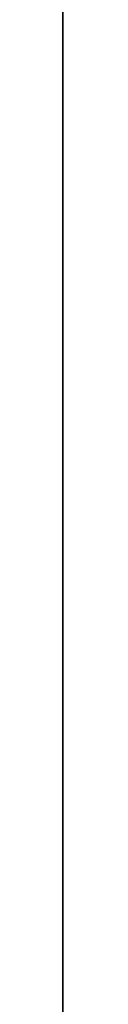
# Model space of a CAD drawing. Units: inches. Extents: x 2083 to 3317, y 1141 to 2115.
# Tile 34 of 256: x 2235.95977 to 2235.95984, y 1477.8005 to 1477.82142. Entities that reach past the tile are written whole.
import ezdxf

# ---------------------------------------------------------------- set-up
doc = ezdxf.new("R2010")
doc.units = ezdxf.units.IN
doc.layers.add('A-ANNO-DIMS', color=2, linetype='Continuous', lineweight=18)
doc.layers.add('A-WALL', color=7, linetype='Continuous', lineweight=35)
doc.layers.add('A-WALL-PATT', color=251, linetype='Continuous', lineweight=13, true_color=0x636466)
doc.styles.get("Standard").update_dxf_attribs({"font": 'arial.ttf'})
doc.dimstyles.new('ISO-25', dxfattribs={"dimtxt": 12, "dimasz": 12, "dimexe": 1.25, "dimexo": 0.625, "dimtad": 1, "dimlunit": 3, "dimtxsty": 'Standard', "dimcen": 2.5, "dimadec": 0, "dimazin": 0, "dimtfac": 1, "dimtmove": 0, "dimatfit": 3, "dimfxl": 1, "dimarcsym": 0})

# ---------------------------------------------------------------- blocks, each defined once
blk = doc.blocks.new('*D30')
at = {"layer": 'A-ANNO-DIMS', "color": 0, "lineweight": -2, "transparency": 16777216}
for p, q in [((2240.017856, 1445.273807), (2240.017856, 1448.045528)), ((2254.329327, 1445.273807), (2254.329327, 1448.045528)), ((2228.017856, 1446.795528), (2216.017856, 1446.795528)), ((2240.017856, 1446.795528), (2254.329327, 1446.795528)), ((2266.329327, 1446.795528), (2413.764866, 1446.795528))]:
    blk.add_line(p, q, dxfattribs=at)
at = {"layer": 'A-ANNO-DIMS', "color": 0, "transparency": 16777216}
for points in [[(2228.017856, 1448.795528), (2228.017856, 1444.795528), (2240.017856, 1446.795528)], [(2266.329327, 1448.795528), (2266.329327, 1444.795528), (2254.329327, 1446.795528)]]:
    blk.add_solid(points, dxfattribs=at)
at = {"layer": 'Defpoints', "color": 0, "transparency": 16777216}
for p in [(2254.329327, 1446.795528), (2240.017856, 1444.648807), (2254.329327, 1444.648807)]:
    blk.add_point(p, dxfattribs=at)
at = {"layer": 'A-ANNO-DIMS', "color": 0, "transparency": 16777216, "insert": (2346.047096, 1453.625167), "char_height": 12, "attachment_point": 5}
blk.add_mtext('WC 1\'-2 1/2" TYP.', dxfattribs=at)
blk = doc.blocks.new('*D31')
at = {"layer": 'A-ANNO-DIMS', "color": 0, "lineweight": -2, "transparency": 16777216}
for p, q in [((2237.871136, 1456.648807), (2237.871136, 1541.915179)), ((2239.392856, 1444.648807), (2236.621136, 1444.648807)), ((2237.871136, 1431.547542), (2237.871136, 1444.648807)), ((2239.392856, 1431.547542), (2236.621136, 1431.547542)), ((2237.871136, 1419.547542), (2237.871136, 1407.547542))]:
    blk.add_line(p, q, dxfattribs=at)
at = {"layer": 'A-ANNO-DIMS', "color": 0, "transparency": 16777216}
for points in [[(2235.871136, 1456.648807), (2239.871136, 1456.648807), (2237.871136, 1444.648807)], [(2235.871136, 1419.547542), (2239.871136, 1419.547542), (2237.871136, 1431.547542)]]:
    blk.add_solid(points, dxfattribs=at)
at = {"layer": 'Defpoints', "color": 0, "transparency": 16777216}
for p in [(2237.871136, 1444.648807), (2240.017856, 1444.648807), (2240.017856, 1431.547542)]:
    blk.add_point(p, dxfattribs=at)
at = {"layer": 'A-ANNO-DIMS', "color": 0, "transparency": 16777216, "insert": (2231.217486, 1505.281993), "char_height": 12, "attachment_point": 5, "rotation": 90}
blk.add_mtext('1\'-1" TYP.', dxfattribs=at)
blk = doc.blocks.new('*D45')
at = {"layer": 'A-ANNO-DIMS', "color": 0, "lineweight": -2, "transparency": 16777216}
for p, q in [((2235.959783, 1478.38636), (2235.959783, 1531.36136)), ((2418.959783, 1478.38636), (2418.959783, 1531.36136)), ((2247.959783, 1530.11136), (2406.959783, 1530.11136))]:
    blk.add_line(p, q, dxfattribs=at)
at = {"layer": 'A-ANNO-DIMS', "color": 0, "transparency": 16777216}
for points in [[(2247.959783, 1532.11136), (2247.959783, 1528.11136), (2235.959783, 1530.11136)], [(2406.959783, 1532.11136), (2406.959783, 1528.11136), (2418.959783, 1530.11136)]]:
    blk.add_solid(points, dxfattribs=at)
at = {"layer": 'Defpoints', "color": 0, "transparency": 16777216}
for p in [(2418.959783, 1530.11136), (2235.959783, 1477.76136), (2418.959783, 1477.76136)]:
    blk.add_point(p, dxfattribs=at)
at = {"layer": 'A-ANNO-DIMS', "color": 0, "transparency": 16777216, "insert": (2327.459783, 1536.867329), "char_height": 12, "attachment_point": 5}
blk.add_mtext('15\'-3"', dxfattribs=at)
blk = doc.blocks.new('*D62')
at = {"layer": 'A-ANNO-DIMS', "color": 0, "lineweight": -2, "transparency": 16777216}
for p, q in [((2235.959783, 1469.38636), (2235.959783, 1522.36136)), ((2379.959783, 1469.38636), (2379.959783, 1522.36136)), ((2247.959783, 1521.11136), (2367.959783, 1521.11136))]:
    blk.add_line(p, q, dxfattribs=at)
at = {"layer": 'A-ANNO-DIMS', "color": 0, "transparency": 16777216}
for points in [[(2247.959783, 1523.11136), (2247.959783, 1519.11136), (2235.959783, 1521.11136)], [(2367.959783, 1523.11136), (2367.959783, 1519.11136), (2379.959783, 1521.11136)]]:
    blk.add_solid(points, dxfattribs=at)
at = {"layer": 'Defpoints', "color": 0, "transparency": 16777216}
for p in [(2379.959783, 1521.11136), (2235.959783, 1468.76136), (2379.959783, 1468.76136)]:
    blk.add_point(p, dxfattribs=at)
at = {"layer": 'A-ANNO-DIMS', "color": 0, "transparency": 16777216, "insert": (2307.959783, 1527.863236), "char_height": 12, "attachment_point": 5}
blk.add_mtext('12\'-0"', dxfattribs=at)

msp = doc.modelspace()

# ---------------------------------------------------------------- hatches: boundary and pattern name
at = {"layer": 'A-WALL-PATT'}
h = msp.add_hatch(color=256, dxfattribs=at)
h.dxf.hatch_style = 1
h.paths.add_polyline_path([(3126.959783, 2020.76136), (2748.959783, 2020.76136), (2604.959783, 2020.76136), (2226.959783, 2020.76136), (2226.959783, 1702.76136), (2466.959783, 1702.76136), (2466.959783, 1582.76136), (2418.959783, 1582.76136), (2418.959783, 1477.76136), (2226.959783, 1477.76136), (2226.959783, 1263.26136), (2544.959783, 1263.26136), (2544.959783, 1411.76136), (2604.959783, 1411.76136), (2685.959783, 1411.76136), (2685.959783, 1420.76136), (2604.959783, 1420.76136), (2604.959783, 1573.76136), (2604.959783, 1702.76136), (2604.959783, 2011.76136), (2748.959783, 2011.76136), (2748.959783, 1702.76136), (2862.959783, 1702.76136), (2862.959783, 1621.76136), (2871.959783, 1621.76136), (2871.959783, 1702.76136), (2883.959783, 1702.76136), (2883.959783, 1706.939459, -0.026459), (2883.959783, 1711.76136), (2757.959783, 1711.76136), (2757.959783, 1807.76136), (2787.959783, 1807.76136), (2787.959783, 1812.26136), (2757.959783, 1812.26136), (2757.959783, 2011.76136), (2877.959783, 2011.76136), (2877.959783, 1812.26136), (2847.959783, 1812.26136), (2847.959783, 1807.76136), (2889.835742, 1807.76136), (2889.835742, 1812.26136), (2882.459783, 1812.26136), (2882.459783, 2011.76136), (3117.959783, 2011.76136), (3117.959783, 1812.26136), (2937.835742, 1812.26136), (2937.835742, 1807.76136), (2995.709783, 1807.76136), (2995.709783, 1796.117666), (3000.209783, 1796.117666), (3000.209783, 1807.76136), (3117.959783, 1807.76136), (3117.959783, 1711.76136), (3000.209783, 1711.76136), (3000.209783, 1760.117666), (2998.572705, 1760.117666, -0.020711), (2995.709783, 1760.117666), (2995.709783, 1711.76136), (2931.959783, 1711.76136), (2931.959783, 1702.76136), (3126.959783, 1702.76136)])
h.paths.add_polyline_path([(2471.459783, 2011.76136), (2471.459783, 1810.01136), (2462.716936, 1810.01136), (2462.716936, 1805.51136), (2505.959783, 1805.51136), (2505.959783, 1810.01136), (2475.959783, 1810.01136), (2475.959783, 2011.76136), (2595.959783, 2011.76136), (2595.959783, 1810.01136), (2565.959783, 1810.01136), (2565.959783, 1805.51136), (2595.959783, 1805.51136), (2595.959783, 1711.76136), (2235.959783, 1711.76136), (2235.959783, 1805.51136), (2353.709783, 1805.51136), (2353.709783, 1796.054162), (2358.209783, 1796.054162), (2358.209783, 1805.51136), (2414.716936, 1805.51136), (2414.716936, 1810.01136), (2235.959783, 1810.01136), (2235.959783, 2011.76136)], flags=16)
h.paths.add_polyline_path([(2270.204734, 1994.610008), (2270.204734, 1970.610008), (2246.204734, 1970.610008), (2246.204734, 1994.610008)], flags=0)
edge = h.paths.add_edge_path(flags=0)
edge.add_ellipse((2332.027391, 1899.798176), major_axis=(-3.042994, 3.042994), ratio=0.16825245, start_angle=-161.332166, end_angle=-156.307114, ccw=False)
edge.add_ellipse((2333.082037, 1898.74353), major_axis=(-1.054646, 1.054646), ratio=0.4535321, start_angle=-123.371019, end_angle=-94.159107)
edge = h.paths.add_edge_path(flags=0)
edge.add_ellipse((2332.027391, 1968.87629), major_axis=(3.042994, 3.042994), ratio=0.16825245, start_angle=18.667834, end_angle=23.692886)
edge.add_spline(control_points=[(2332.925596, 1970.691105), (2332.226768, 1970.3361), (2330.893709, 1969.658905), (2328.41308, 1970.932138), (2327.203934, 1967.748712), (2324.709596, 1969.955589), (2322.532822, 1967.012354), (2320.012846, 1971.295812), (2317.680308, 1968.157845), (2316.040526, 1967.102047), (2315.426904, 1966.809602)], knot_values=[0, 0, 0, 0, 2.267059, 4.324559, 6.685584, 8.878641, 11.121502, 14.300359, 17.755284, 19.732645, 19.732645, 19.732645, 19.732645], degree=3, periodic=0)
edge.add_ellipse((2332.027391, 1968.87629), major_axis=(3.042994, 3.042994), ratio=0.16825245, start_angle=18.667834, end_angle=23.692886, ccw=False)
edge.add_ellipse((2333.082037, 1969.930936), major_axis=(1.054646, 1.054646), ratio=0.4535321, start_angle=56.628981, end_angle=85.840893, ccw=False)
edge = h.paths.add_edge_path(flags=0)
edge.add_spline(control_points=[(2296.428287, 1967.987908), (2293.627804, 1965.336314), (2287.703624, 1959.727094), (2299.74386, 1949.995699), (2294.532591, 1935.668528), (2290.573228, 1920.603512), (2293.394124, 1909.973691), (2296.185407, 1904.966543)], knot_values=[0.099185, 0.099185, 0.099185, 0.099185, 0.345301, 0.619822, 0.982653, 1.386093, 1.810555, 1.810555, 1.810555, 1.810555], degree=3, periodic=0)
edge.add_spline(control_points=[(2296.185407, 1904.966543), (2297.383582, 1902.6193), (2298.000969, 1901.949312), (2298.55297, 1901.468155)], knot_values=[0.006246, 0.006246, 0.006246, 0.006246, 0.055476, 0.055476, 0.055476, 0.055476], degree=3, periodic=0)
edge.add_spline(control_points=[(2298.55297, 1901.468155), (2297.258612, 1900.923224), (2295.225294, 1900.232126), (2293.060229, 1900.614205), (2292.101423, 1900.788415), (2292.089578, 1900.790568)], knot_values=[0.312835, 0.312835, 0.312835, 0.312835, 0.40178, 0.474987, 0.475903, 0.475903, 0.475903, 0.475903], degree=3, periodic=0)
edge.add_arc((2292.793646, 1904.664109), 3.937008, 215.420897, 259.698179, ccw=False)
edge.add_spline(control_points=[(2289.585314, 1902.382304), (2289.476652, 1902.535087), (2289.36848, 1902.688035), (2289.260865, 1902.84117)], knot_values=[0.102872, 0.102872, 0.102872, 0.102872, 0.116896, 0.116896, 0.116896, 0.116896], degree=3, periodic=0)
edge.add_spline(control_points=[(2289.260865, 1902.84117), (2288.686604, 1902.550192), (2287.640048, 1902.019902), (2285.881337, 1901.873954), (2283.852972, 1901.504352), (2281.719987, 1899.710538), (2278.466991, 1899.492942), (2276.157136, 1901.883202), (2272.258953, 1899.804071), (2267.777605, 1901.843183), (2262.243882, 1900.184033), (2257.414927, 1901.782061), (2254.318374, 1900.72612), (2253.178285, 1900.337343)], knot_values=[0, 0, 0, 0, 1.907977, 3.477176, 5.261074, 7.972851, 11.680248, 13.717921, 16.939592, 22.789562, 27.502503, 33.595215, 37.145618, 37.145618, 37.145618, 37.145618], degree=3, periodic=0)
edge.add_line((2253.178285, 1900.337343), (2250.24424, 1902.84117))
edge.add_line((2250.24424, 1902.84117), (2250.24424, 1965.833296))
edge.add_line((2250.24424, 1965.833296), (2253.178285, 1968.337123))
edge.add_spline(control_points=[(2253.178285, 1968.337123), (2254.318374, 1967.948346), (2257.414927, 1966.892405), (2262.243882, 1968.490433), (2267.777605, 1966.831283), (2271.52673, 1968.537217), (2273.875914, 1967.828289), (2274.206701, 1967.727642)], knot_values=[0, 0, 0, 0, 0.09018, 0.244935, 0.364644, 0.513233, 0.537855, 0.537855, 0.537855, 0.537855], degree=3, periodic=0)
edge.add_arc((2274.352887, 1963.793349), 3.937008, 72.051134, 92.127949, ccw=False)
edge.add_arc((2281.296933, 1985.230003), 18.596298, 252.0511336, 288.5657217)
edge.add_arc((2292.316717, 1956.02888), 12.646081, 71.0267879, 113.7782184, ccw=False)
edge = h.paths.add_edge_path(flags=0)
edge.add_spline(control_points=[(2274.899415, 1951.856195), (2275.066156, 1951.616592), (2275.232687, 1951.376588), (2275.397987, 1951.135855)], knot_values=[1.409916, 1.409916, 1.409916, 1.409916, 1.43159, 1.43159, 1.43159, 1.43159], degree=3, periodic=0)
edge.add_spline(control_points=[(2275.397987, 1951.135855), (2275.792106, 1950.561885), (2276.179231, 1949.983774), (2276.545546, 1949.397103)], knot_values=[1.358238, 1.358238, 1.358238, 1.358238, 1.409916, 1.409916, 1.409916, 1.409916], degree=3, periodic=0)
edge.add_line((2276.545546, 1949.397103), (2277.437289, 1947.862185))
edge.add_spline(control_points=[(2277.437289, 1947.862185), (2276.303834, 1945.673115), (2274.639698, 1942.426882), (2274.631615, 1938.0939), (2272.799124, 1930.85155), (2274.356426, 1943.897046), (2275.947681, 1947.923356), (2276.545546, 1949.397103)], knot_values=[0.005632, 0.005632, 0.005632, 0.005632, 0.186014, 0.266002, 0.357087, 0.59639, 0.739732, 0.739732, 0.739732, 0.739732], degree=3, periodic=0)
edge.add_spline(control_points=[(2276.545546, 1949.397103), (2276.179231, 1949.983774), (2275.792106, 1950.561885), (2275.397987, 1951.135855)], knot_values=[1.358238, 1.358238, 1.358238, 1.358238, 1.409916, 1.409916, 1.409916, 1.409916], degree=3, periodic=0)
edge.add_spline(control_points=[(2275.397987, 1951.135855), (2274.9425, 1950.080452), (2274.20776, 1948.025272), (2273.934602, 1944.851477), (2272.468534, 1937.627489), (2273.466216, 1945.696466), (2274.700615, 1951.059472), (2274.899415, 1951.856195)], knot_values=[0.104364, 0.104364, 0.104364, 0.104364, 0.189636, 0.269624, 0.36071, 0.600013, 0.644622, 0.644622, 0.644622, 0.644622], degree=3, periodic=0)
h.paths.add_polyline_path([(2269.167514, 1963.127573, -0.357527), (2268.170633, 1960.97637, -0.092561), (2268.170633, 1939.436325, -0.357527), (2269.167514, 1937.285122, -0.357527), (2267.01631, 1938.282002, -0.164785), (2254.685581, 1938.282002, -0.357527), (2252.534378, 1937.285122, -0.357527), (2253.531259, 1939.436325, -0.092561), (2253.531259, 1960.97637, -0.357527), (2252.534378, 1963.127573, -0.357527), (2254.685581, 1962.130692, -0.164785), (2267.01631, 1962.130692, -0.357527)], flags=0)
h.paths.add_polyline_path([(2248.874068, 1967.8018), (2248.874068, 1957.02771), (2249.457783, 1957.02771), (2249.457783, 1911.646756), (2248.874068, 1911.646756), (2248.874068, 1900.872666), (2246.511863, 1900.872666, 0.197327), (2244.149658, 1902.456873), (2244.149658, 1966.217592, 0.197327), (2246.511863, 1967.8018)], flags=0)
h.paths.add_polyline_path([(2269.167514, 1931.389344, -0.357527), (2268.170633, 1929.238141, -0.092561), (2268.170633, 1907.698096, -0.357527), (2269.167514, 1905.546893, -0.357527), (2267.01631, 1906.543774, -0.164785), (2254.685581, 1906.543774, -0.357527), (2252.534378, 1905.546893, -0.357527), (2253.531259, 1907.698096, -0.092561), (2253.531259, 1929.238141, -0.357527), (2252.534378, 1931.389344, -0.357527), (2254.685581, 1930.392463, -0.164785), (2267.01631, 1930.392463, -0.357527)], flags=0)
edge = h.paths.add_edge_path(flags=0)
edge.add_spline(control_points=[(2276.196858, 1906.723702), (2276.168144, 1909.028928), (2276.114049, 1913.371852), (2270.598417, 1924.924978), (2273.905175, 1919.012779), (2275.921711, 1916.262063), (2275.47457, 1912.402149), (2277.257874, 1910.380621), (2276.696044, 1908.225036), (2276.646218, 1906.813023), (2276.617825, 1906.008407)], knot_values=[0, 0, 0, 0, 8.61026, 16.221274, 18.843057, 23.804898, 27.440828, 29.356102, 31.203478, 33.650687, 33.650687, 33.650687, 33.650687], degree=3, periodic=0)
edge.add_spline(control_points=[(2276.617825, 1906.008407), (2276.623313, 1905.624144), (2276.497738, 1904.628661), (2275.441779, 1903.854725), (2274.937314, 1903.08045), (2274.85908, 1902.84117)], knot_values=[0.156488, 0.156488, 0.156488, 0.156488, 0.184398, 0.231376, 0.250598, 0.250598, 0.250598, 0.250598], degree=3, periodic=0)
edge.add_line((2274.85908, 1902.84117), (2276.50598, 1902.84117))
edge.add_spline(control_points=[(2276.50598, 1902.84117), (2276.788308, 1903.08494), (2277.665071, 1904.125196), (2278.249538, 1904.340738), (2277.653872, 1908.527387), (2278.15567, 1906.227808), (2278.100464, 1905.285948), (2278.846675, 1904.069005), (2277.856785, 1903.414948), (2277.874191, 1902.99105), (2277.903562, 1902.84117)], knot_values=[0.059574, 0.059574, 0.059574, 0.059574, 0.080753, 0.103741, 0.16972, 0.176036, 0.207137, 0.240474, 0.262341, 0.27366, 0.27366, 0.27366, 0.27366], degree=3, periodic=0)
edge.add_line((2277.903562, 1902.84117), (2280.029825, 1902.84117))
edge.add_spline(control_points=[(2280.029825, 1902.84117), (2279.888221, 1903.088398), (2279.499257, 1903.981551), (2280.152284, 1905.939349), (2278.103615, 1909.657757), (2279.762395, 1907.185285), (2280.3279, 1904.874861), (2280.485109, 1903.48959), (2281.463269, 1903.249432), (2281.758343, 1902.936497), (2281.834036, 1902.84117)], knot_values=[0.013856, 0.013856, 0.013856, 0.013856, 0.034874, 0.088867, 0.107879, 0.126738, 0.158714, 0.193757, 0.217487, 0.226722, 0.226722, 0.226722, 0.226722], degree=3, periodic=0)
edge.add_spline(control_points=[(2281.834036, 1902.84117), (2281.787535, 1902.826703), (2281.647022, 1902.782988), (2281.395527, 1902.85949), (2281.088077, 1902.985242), (2280.720683, 1903.060902), (2280.333451, 1903.025726), (2280.124767, 1902.898879), (2280.029825, 1902.84117)], knot_values=[0, 0, 0, 0, 0.14413, 0.435517, 0.749276, 1.153046, 1.548371, 1.878348, 1.878348, 1.878348, 1.878348], degree=3, periodic=0)
edge.add_line((2280.029825, 1902.84117), (2277.903562, 1902.84117))
edge.add_spline(control_points=[(2277.903562, 1902.84117), (2277.892855, 1902.795855), (2277.865396, 1902.679637), (2277.607479, 1902.687483), (2277.27405, 1902.8007), (2276.837921, 1902.619775), (2276.583807, 1902.789261), (2276.50598, 1902.84117)], knot_values=[0, 0, 0, 0, 0.127189, 0.326199, 0.628009, 1.24357, 1.515331, 1.515331, 1.515331, 1.515331], degree=3, periodic=0)
edge.add_line((2276.50598, 1902.84117), (2274.85908, 1902.84117))
edge.add_spline(control_points=[(2274.85908, 1902.84117), (2274.814437, 1902.898587), (2274.72513, 1903.013446), (2274.493477, 1903.118968), (2274.244285, 1902.960539), (2273.937121, 1903.184942), (2273.614039, 1902.983143), (2273.408316, 1902.883045), (2273.322254, 1902.84117)], knot_values=[0, 0, 0, 0, 0.21843, 0.436957, 0.687977, 0.990379, 1.398396, 1.69185, 1.69185, 1.69185, 1.69185], degree=3, periodic=0)
edge.add_spline(control_points=[(2273.322254, 1902.84117), (2273.61674, 1903.445692), (2274.273998, 1904.538253), (2276.027239, 1904.573702), (2276.206963, 1906.583637), (2276.196858, 1906.723702)], knot_values=[0.012227, 0.012227, 0.012227, 0.012227, 0.059472, 0.106218, 0.134458, 0.134458, 0.134458, 0.134458], degree=3, periodic=0)
h.paths.add_polyline_path([(2270.776054, 1897.789828), (2270.776054, 1873.789828), (2246.776054, 1873.789828), (2246.776054, 1897.789828)], flags=0)
h.paths.add_polyline_path([(2353.709783, 1760.005059), (2353.709783, 1760.054162), (2358.209783, 1760.054162, -0.033729)], flags=0)
h.paths.add_polyline_path([(2321.819119, 1737.529186), (2341.995327, 1737.529186, -0.414214), (2343.203273, 1736.321241), (2343.203273, 1721.020596, -0.414214), (2341.995327, 1719.812651), (2321.819119, 1719.812651, -0.414214), (2320.611173, 1721.020596), (2320.611173, 1736.321241, -0.414214)], flags=0)
h.paths.add_polyline_path([(2324.23501, 1736.321241), (2339.579436, 1736.321241, -0.414214), (2341.995327, 1733.905349), (2341.995327, 1725.44973, -0.414214), (2339.579436, 1723.033839), (2333.680588, 1723.033839), (2333.845317, 1722.045467, -0.870646), (2335.425399, 1721.825893, -0.767327), (2333.922694, 1721.423245), (2331.291024, 1721.423245, -0.767327), (2329.788319, 1721.825893, -0.870646), (2331.368401, 1722.045467), (2331.53313, 1723.033839), (2324.23501, 1723.033839, -0.414214), (2321.819119, 1725.44973), (2321.819119, 1733.905349, -0.414214)], flags=0)
h.paths.add_polyline_path([(2570.483789, 1928.615444), (2589.683789, 1928.615444), (2590.168829, 1928.615444), (2590.168829, 1904.993397), (2570.483789, 1904.993397)], flags=0)
h.paths.add_polyline_path([(2574.447324, 1927.263822, -1), (2572.828836, 1927.263822, -1)], flags=0)
h.paths.add_polyline_path([(2573.089867, 1926.940877), (2573.925032, 1927.776042), (2574.147743, 1927.553332), (2573.312577, 1926.718166)], flags=0)
h.paths.add_polyline_path([(2578.779065, 1919.729618, -1), (2571.591663, 1919.729618, -1)], flags=0)
h.paths.add_polyline_path([(2578.385364, 1919.729618, -1), (2571.985364, 1919.729618, -1)], flags=0)
h.paths.add_polyline_path([(2331.595764, 1729.476216, -1), (2333.617954, 1729.476216, -1)], flags=0)
h.paths.add_polyline_path([(2578.034228, 1927.263822, -1), (2576.41574, 1927.263822, -1)], flags=0)
h.paths.add_polyline_path([(2576.688851, 1927.531089), (2576.911562, 1927.753799), (2577.746728, 1926.918634), (2577.524017, 1926.695923)], flags=0)
h.paths.add_polyline_path([(2578.139065, 1909.859539, -1), (2572.231663, 1909.859539, -1)], flags=0)
h.paths.add_polyline_path([(2577.745364, 1909.859539, -1), (2572.625364, 1909.859539, -1)], flags=0)
h.paths.add_polyline_path([(2583.797718, 1927.263822, -1), (2582.179229, 1927.263822, -1)], flags=0)
h.paths.add_polyline_path([(2582.718649, 1927.753799), (2583.553814, 1926.918634), (2583.331103, 1926.695923), (2582.495938, 1927.531089)], flags=0)
h.paths.add_polyline_path([(2582.495938, 1927.531089), (2582.718649, 1927.753799), (2583.553814, 1926.918634), (2583.331103, 1926.695923)], flags=0)
h.paths.add_polyline_path([(2587.739065, 1920.529618, -1), (2581.831663, 1920.529618, -1)], flags=0)
h.paths.add_polyline_path([(2587.345364, 1920.529618, -1), (2582.225364, 1920.529618, -1)], flags=0)
h.paths.add_polyline_path([(2587.384622, 1927.263822, -1), (2585.766133, 1927.263822, -1)], flags=0)
h.paths.add_polyline_path([(2586.081993, 1926.980247), (2586.917158, 1927.815412), (2587.139869, 1927.592702), (2586.304703, 1926.757536)], flags=0)
h.paths.add_polyline_path([(2588.379065, 1910.659539, -1), (2581.191663, 1910.659539, -1)], flags=0)
h.paths.add_polyline_path([(2587.985364, 1910.659539, -1), (2581.585364, 1910.659539, -1)], flags=0)
h.paths.add_polyline_path([(2417.167729, 1729.477895), (2437.343937, 1729.477895, -0.414214), (2438.551883, 1728.26995), (2438.551883, 1712.969306, -0.414214), (2437.343937, 1711.76136), (2417.167729, 1711.76136, -0.414214), (2415.959783, 1712.969306), (2415.959783, 1728.26995, -0.414214)], flags=0)
h.paths.add_polyline_path([(2419.58362, 1728.26995), (2434.928046, 1728.26995, -0.414214), (2437.343937, 1725.854059), (2437.343937, 1717.39844, -0.414214), (2434.928046, 1714.982548), (2429.029199, 1714.982548), (2429.193927, 1713.994176, -0.870646), (2430.774009, 1713.774603, -0.767327), (2429.271304, 1713.371954), (2426.639634, 1713.371954, -0.767327), (2425.136929, 1713.774603, -0.870646), (2426.717011, 1713.994176), (2426.88174, 1714.982548), (2419.58362, 1714.982548, -0.414214), (2417.167729, 1717.39844), (2417.167729, 1725.854059, -0.414214)], flags=0)
h.paths.add_polyline_path([(2419.58362, 1728.26995), (2434.928046, 1728.26995, -0.414214), (2437.343937, 1725.854059), (2437.343937, 1717.39844, -0.414214), (2434.928046, 1714.982548), (2429.029199, 1714.982548), (2428.358118, 1719.009034), (2427.552821, 1719.009034), (2426.88174, 1714.982548), (2419.58362, 1714.982548, -0.414214), (2417.167729, 1717.39844), (2417.167729, 1725.854059, -0.414214)], flags=0)
h.paths.add_polyline_path([(2426.944374, 1721.424925, -1), (2428.966564, 1721.424925, -1)], flags=0)
h.paths.add_polyline_path([(2475.959783, 1702.76136), (2595.959783, 1702.76136), (2595.959783, 1582.76136), (2475.959783, 1582.76136)], flags=16)
h.paths.add_polyline_path([(2427.959783, 1573.76136), (2595.959783, 1573.76136), (2595.959783, 1468.76136), (2595.959783, 1420.76136), (2384.459783, 1420.76136), (2384.459783, 1468.76136), (2427.959783, 1468.76136)], flags=16)
h.paths.add_polyline_path([(2379.959783, 1468.76136), (2379.959783, 1420.76136), (2235.959783, 1420.76136), (2235.959783, 1468.76136)], flags=16)
h.paths.add_polyline_path([(2317.815996, 1466.695767), (2337.992205, 1466.695767, -0.414214), (2339.20015, 1465.487821), (2339.20015, 1450.187177, -0.414214), (2337.992205, 1448.979232), (2317.815996, 1448.979232, -0.414214), (2316.608051, 1450.187177), (2316.608051, 1465.487821, -0.414214)], flags=0)
h.paths.add_polyline_path([(2320.231887, 1465.487821), (2335.576313, 1465.487821, -0.414214), (2337.992205, 1463.07193), (2337.992205, 1454.616311, -0.414214), (2335.576313, 1452.20042), (2329.677466, 1452.20042), (2329.842195, 1451.212047, -0.870646), (2331.422276, 1450.992474, -0.767327), (2329.919571, 1450.589826), (2327.287902, 1450.589826, -0.767327), (2325.785197, 1450.992474, -0.870646), (2327.365278, 1451.212047), (2327.530007, 1452.20042), (2320.231887, 1452.20042, -0.414214), (2317.815996, 1454.616311), (2317.815996, 1463.07193, -0.414214)], flags=0)
h.paths.add_polyline_path([(2320.231887, 1465.487821), (2335.576313, 1465.487821, -0.414214), (2337.992205, 1463.07193), (2337.992205, 1454.616311, -0.414214), (2335.576313, 1452.20042), (2329.677466, 1452.20042), (2329.006385, 1456.226905), (2328.201088, 1456.226905), (2327.530007, 1452.20042), (2320.231887, 1452.20042, -0.414214), (2317.815996, 1454.616311), (2317.815996, 1463.07193, -0.414214)], flags=0)
h.paths.add_polyline_path([(2327.592641, 1458.642796, -1), (2329.614832, 1458.642796, -1)], flags=0)
h.paths.add_polyline_path([(2244.411744, 1433.340453), (2241.920945, 1433.340453, -0.414214), (2240.017856, 1435.243542), (2240.017856, 1440.952808, -0.414211), (2241.920925, 1442.855897), (2244.411744, 1442.855897, -1.976472)], flags=0)
h.paths.add_polyline_path([(2245.356888, 1434.397536, -0.414214), (2245.356888, 1441.798814, -2.144098)], flags=0)
h.paths.add_polyline_path([(2535.959783, 1416.26136), (2535.959783, 1272.26136), (2235.959783, 1272.26136), (2235.959783, 1416.26136)], flags=16)
h.paths.add_polyline_path([(2260.119561, 1384.292841), (2260.119561, 1362.038649), (2237.865369, 1362.038649), (2237.865369, 1384.292841)], flags=0)
edge = h.paths.add_edge_path(flags=0)
edge.add_line((2318.251847, 1362.093298), (2318.145797, 1362.000973))
edge.add_ellipse((2317.445116, 1360.431044), major_axis=(2.82164, 2.82164), ratio=0.16825245, start_angle=18.667834, end_angle=20.948127, ccw=False)
edge.add_ellipse((2318.423045, 1361.408974), major_axis=(0.977929, 0.977929), ratio=0.4535321, start_angle=56.628981, end_angle=70.226201, ccw=False)
edge = h.paths.add_edge_path(flags=0)
edge.add_line((2319.10737, 1295.571078), (2319.015044, 1295.677128))
edge.add_ellipse((2317.445116, 1296.377809), major_axis=(-2.82164, 2.82164), ratio=0.16825245, start_angle=-161.332166, end_angle=-159.051873, ccw=False)
edge.add_ellipse((2318.423045, 1295.39988), major_axis=(-0.977929, 0.977929), ratio=0.4535321, start_angle=-123.371019, end_angle=-109.773799)
edge = h.paths.add_edge_path(flags=0)
edge.add_spline(control_points=[(2284.210349, 1301.170219), (2284.580688, 1300.444719), (2284.891189, 1299.892024), (2285.159553, 1299.461018)], knot_values=[0.039066, 0.039066, 0.039066, 0.039066, 0.055476, 0.055476, 0.055476, 0.055476], degree=3, periodic=0)
edge.add_line((2285.159553, 1299.461018), (2284.210349, 1301.170219))
edge = h.paths.add_edge_path(flags=0)
edge.add_line((2280.412458, 1297.298013), (2283.369991, 1297.036122))
edge.add_line((2283.369991, 1297.036122), (2286.40569, 1297.92631))
edge.add_spline(control_points=[(2286.40569, 1297.92631), (2285.305487, 1297.463119), (2284.344777, 1297.129151), (2283.369991, 1297.036122)], knot_values=[0.394369, 0.394369, 0.394369, 0.394369, 0.475903, 0.475903, 0.475903, 0.475903], degree=3, periodic=0)
edge.add_spline(control_points=[(2283.369991, 1297.036122), (2283.28139, 1297.027666), (2282.316289, 1296.957336), (2281.312502, 1297.134479), (2280.423441, 1297.296016), (2280.412458, 1297.298013)], knot_values=[0.312835, 0.312835, 0.312835, 0.312835, 0.320246, 0.393453, 0.394369, 0.394369, 0.394369, 0.394369], degree=3, periodic=0)
edge = h.paths.add_edge_path(flags=0)
edge.add_line((2284.435561, 1359.607285), (2280.446291, 1355.328047))
edge.add_line((2280.446291, 1355.328047), (2279.579987, 1351.017754))
edge.add_line((2279.579987, 1351.017754), (2282.412974, 1346.580433))
edge.add_spline(control_points=[(2282.412974, 1346.580433), (2283.153331, 1345.589236), (2284.252896, 1344.028897), (2284.801037, 1342.387167), (2284.935162, 1341.805544)], knot_values=[1.240098, 1.240098, 1.240098, 1.240098, 1.332892, 1.382712, 1.382712, 1.382712, 1.382712], degree=3, periodic=0)
edge.add_spline(control_points=[(2284.935162, 1341.805544), (2285.319108, 1340.1406), (2285.233029, 1338.409204), (2284.909938, 1336.654122)], knot_values=[1.097484, 1.097484, 1.097484, 1.097484, 1.240098, 1.240098, 1.240098, 1.240098], degree=3, periodic=0)
edge.add_spline(control_points=[(2284.909938, 1336.654122), (2284.586848, 1334.89904), (2284.026745, 1333.120272), (2283.462644, 1331.360585)], knot_values=[0.95487, 0.95487, 0.95487, 0.95487, 1.097484, 1.097484, 1.097484, 1.097484], degree=3, periodic=0)
edge.add_line((2283.462644, 1331.360585), (2281.890376, 1326.153357))
edge.add_line((2281.890376, 1326.153357), (2280.756259, 1321.056089))
edge.add_line((2280.756259, 1321.056089), (2280.299205, 1316.001977))
edge.add_line((2280.299205, 1316.001977), (2280.715933, 1310.950068))
edge.add_line((2280.715933, 1310.950068), (2282.028094, 1305.972137))
edge.add_line((2282.028094, 1305.972137), (2284.210349, 1301.170219))
edge.add_spline(control_points=[(2284.210349, 1301.170219), (2283.340731, 1302.730185), (2282.611904, 1304.336493), (2282.028094, 1305.972137)], knot_values=[0.099185, 0.099185, 0.099185, 0.099185, 0.241799, 0.241799, 0.241799, 0.241799], degree=3, periodic=0)
edge.add_spline(control_points=[(2282.028094, 1305.972137), (2281.444283, 1307.60778), (2281.005489, 1309.272759), (2280.715933, 1310.950068)], knot_values=[0.241799, 0.241799, 0.241799, 0.241799, 0.384413, 0.384413, 0.384413, 0.384413], degree=3, periodic=0)
edge.add_spline(control_points=[(2280.715933, 1310.950068), (2280.433241, 1312.587613), (2280.289386, 1314.276959), (2280.298894, 1315.962032), (2280.299205, 1316.001977)], knot_values=[0.384413, 0.384413, 0.384413, 0.384413, 0.523647, 0.527028, 0.527028, 0.527028, 0.527028], degree=3, periodic=0)
edge.add_spline(control_points=[(2280.299205, 1316.001977), (2280.312326, 1317.686955), (2280.477871, 1319.367926), (2280.756259, 1321.056089)], knot_values=[0.527028, 0.527028, 0.527028, 0.527028, 0.669642, 0.669642, 0.669642, 0.669642], degree=3, periodic=0)
edge.add_spline(control_points=[(2280.756259, 1321.056089), (2281.034648, 1322.744252), (2281.42588, 1324.439608), (2281.890376, 1326.153357)], knot_values=[0.669642, 0.669642, 0.669642, 0.669642, 0.812256, 0.812256, 0.812256, 0.812256], degree=3, periodic=0)
edge.add_spline(control_points=[(2281.890376, 1326.153357), (2282.264383, 1327.533251), (2282.78787, 1329.26181), (2283.352751, 1331.01778), (2283.462644, 1331.360585)], knot_values=[0.812256, 0.812256, 0.812256, 0.812256, 0.927087, 0.95487, 0.95487, 0.95487, 0.95487], degree=3, periodic=0)
edge.add_line((2283.462644, 1331.360585), (2284.909938, 1336.654122))
edge.add_line((2284.909938, 1336.654122), (2284.935162, 1341.805544))
edge.add_line((2284.935162, 1341.805544), (2282.412974, 1346.580433))
edge.add_spline(control_points=[(2282.412974, 1346.580433), (2281.275127, 1348.103792), (2280.078447, 1349.570318), (2279.579987, 1351.017754)], knot_values=[1.382712, 1.382712, 1.382712, 1.382712, 1.525326, 1.525326, 1.525326, 1.525326], degree=3, periodic=0)
edge.add_spline(control_points=[(2279.579987, 1351.017754), (2279.443282, 1351.414721), (2279.136312, 1352.856922), (2279.73519, 1354.290385), (2280.446291, 1355.328047)], knot_values=[1.525326, 1.525326, 1.525326, 1.525326, 1.564439, 1.667941, 1.667941, 1.667941, 1.667941], degree=3, periodic=0)
edge.add_spline(control_points=[(2280.446291, 1355.328047), (2281.426113, 1356.757835), (2282.930837, 1358.18256), (2284.435561, 1359.607285)], knot_values=[1.667941, 1.667941, 1.667941, 1.667941, 1.810555, 1.810555, 1.810555, 1.810555], degree=3, periodic=0)
edge.add_arc((2280.623075, 1348.518181), 11.72618, 71.0267879, 113.7782184)
edge.add_arc((2270.404892, 1375.595156), 17.243567, 252.0511336, 288.5657217, ccw=False)
edge.add_arc((2263.965969, 1355.717847), 3.650622, 72.051134, 92.127949)
edge.add_arc((2263.965969, 1355.717847), 3.650622, 92.127949, 177.98513)
edge.add_spline(control_points=[(2260.317604, 1355.846199), (2260.260417, 1354.220668), (2260.551278, 1350.186547), (2262.999344, 1346.766251), (2264.472741, 1344.649024)], knot_values=[1.43159, 1.43159, 1.43159, 1.43159, 1.564144, 1.770695, 1.770695, 1.770695, 1.770695], degree=3, periodic=0)
edge.add_line((2264.472741, 1344.649024), (2264.93559, 1343.98253))
edge.add_spline(control_points=[(2263.801044, 1340.248105), (2263.843238, 1340.514088), (2264.067244, 1341.756465), (2264.512693, 1343.002453), (2264.935047, 1343.981083)], knot_values=[0.53657, 0.53657, 0.53657, 0.53657, 0.559349, 0.644622, 0.644622, 0.644622, 0.644622], degree=3, periodic=0)
edge.add_spline(control_points=[(2264.935047, 1343.981083), (2265.117771, 1343.714975), (2265.298875, 1343.447906), (2265.476756, 1343.179365)], knot_values=[1.384077, 1.384077, 1.384077, 1.384077, 1.409916, 1.409916, 1.409916, 1.409916], degree=3, periodic=0)
edge.add_spline(control_points=[(2265.476756, 1343.179365), (2265.654637, 1342.910823), (2265.829296, 1342.64081), (2265.99913, 1342.368812)], knot_values=[1.358238, 1.358238, 1.358238, 1.358238, 1.384077, 1.384077, 1.384077, 1.384077], degree=3, periodic=0)
edge.add_line((2265.99913, 1342.368812), (2266.826006, 1340.945547))
edge.add_spline(control_points=[(2266.826006, 1340.945547), (2268.894401, 1337.089691), (2271.398173, 1325.843001), (2270.516164, 1310.568557), (2275.919376, 1301.860609), (2277.789511, 1299.19945)], knot_values=[0.116896, 0.116896, 0.116896, 0.116896, 0.472987, 1.050969, 1.313793, 1.313793, 1.313793, 1.313793], degree=3, periodic=0)
edge.add_spline(control_points=[(2277.789511, 1299.19945), (2277.839405, 1299.128452), (2277.889428, 1299.057498), (2277.939572, 1298.986584)], knot_values=[0.109884, 0.109884, 0.109884, 0.109884, 0.116896, 0.116896, 0.116896, 0.116896], degree=3, periodic=0)
edge.add_line((2277.939572, 1298.986584), (2277.788849, 1299.199114))
edge.add_spline(control_points=[(2277.788849, 1299.199114), (2277.256582, 1298.929414), (2276.28635, 1298.437902), (2275.039352, 1298.334419), (2274.38333, 1298.238895), (2274.215254, 1298.209338)], knot_values=[33.12187, 33.12187, 33.12187, 33.12187, 35.029056, 36.598255, 37.144827, 37.144827, 37.144827, 37.144827], degree=3, periodic=0)
edge.add_line((2274.215254, 1298.209338), (2273.073147, 1297.892961))
edge.add_spline(control_points=[(2273.073147, 1297.892961), (2272.322936, 1297.579784), (2271.039151, 1296.510508), (2269.248395, 1296.226062), (2268.4231, 1296.374654)], knot_values=[26.532584, 26.532584, 26.532584, 26.532584, 29.198919, 31.839101, 31.839101, 31.839101, 31.839101], degree=3, periodic=0)
edge.add_line((2268.4231, 1296.374654), (2263.878501, 1297.457534))
edge.add_spline(control_points=[(2263.878501, 1297.457534), (2263.556077, 1297.359435), (2261.860306, 1296.838694), (2260.23878, 1297.282407), (2258.933454, 1297.516461)], knot_values=[15.919551, 15.919551, 15.919551, 15.919551, 16.939592, 21.226067, 21.226067, 21.226067, 21.226067], degree=3, periodic=0)
edge.add_line((2258.933454, 1297.516461), (2254.055233, 1297.32901))
edge.add_spline(control_points=[(2254.055233, 1297.32901), (2253.755525, 1297.295815), (2252.113683, 1297.165174), (2250.461869, 1297.544221), (2249.129686, 1297.667882)], knot_values=[5.306517, 5.306517, 5.306517, 5.306517, 6.276435, 10.613034, 10.613034, 10.613034, 10.613034], degree=3, periodic=0)
edge.add_line((2249.129686, 1297.667882), (2244.33165, 1296.877756))
edge.add_line((2244.33165, 1296.877756), (2241.611033, 1299.19945))
edge.add_line((2241.611033, 1299.19945), (2241.611033, 1357.609404))
edge.add_line((2241.611033, 1357.609404), (2244.33165, 1359.931097))
edge.add_line((2244.33165, 1359.931097), (2252.728823, 1359.542692))
edge.add_spline(control_points=[(2252.728823, 1359.542692), (2252.870939, 1359.54644), (2253.30574, 1359.548172), (2253.739845, 1359.514274), (2254.031742, 1359.482426)], knot_values=[0.233291, 0.233291, 0.233291, 0.233291, 0.244935, 0.268927, 0.268927, 0.268927, 0.268927], degree=3, periodic=0)
edge.add_line((2254.031742, 1359.482426), (2259.58719, 1359.41639))
edge.add_spline(control_points=[(2259.58719, 1359.41639), (2260.677068, 1359.628503), (2262.073197, 1359.897003), (2263.523692, 1359.459278), (2263.830417, 1359.365952)], knot_values=[0.422516, 0.422516, 0.422516, 0.422516, 0.513233, 0.537855, 0.537855, 0.537855, 0.537855], degree=3, periodic=0)
edge.add_arc((2263.965969, 1355.717847), 3.650622, 72.051134, 92.127949, ccw=False)
edge.add_arc((2270.404892, 1375.595156), 17.243567, 252.0511336, 288.5657217)
edge.add_arc((2280.623075, 1348.518181), 11.72618, 71.0267879, 113.7782184, ccw=False)
h.paths.add_polyline_path([(2240.34053, 1359.434715), (2240.34053, 1349.444353), (2240.881785, 1349.444353), (2240.881785, 1307.3645), (2240.34053, 1307.3645), (2240.34053, 1297.374138), (2238.150157, 1297.374138, 0.197327), (2235.959783, 1298.843108), (2235.959783, 1357.965746, 0.197327), (2238.150157, 1359.434715)], flags=0)
h.paths.add_polyline_path([(2259.15779, 1355.1005, -0.357527), (2258.233425, 1353.10578, -0.092561), (2258.233425, 1333.132601, -0.357527), (2259.15779, 1331.13788, -0.357527), (2257.16307, 1332.062246, -0.164785), (2245.729302, 1332.062246, -0.357527), (2243.734582, 1331.13788, -0.357527), (2244.658947, 1333.132601, -0.092561), (2244.658947, 1353.10578, -0.357527), (2243.734582, 1355.1005, -0.357527), (2245.729302, 1354.176135, -0.164785), (2257.16307, 1354.176135, -0.357527)], flags=0)
edge = h.paths.add_edge_path(flags=0)
edge.add_line((2265.99913, 1342.368812), (2266.826006, 1340.945547))
edge.add_line((2266.826006, 1340.945547), (2265.307557, 1337.814066))
edge.add_line((2265.307557, 1337.814066), (2264.358232, 1334.652939))
edge.add_line((2264.358232, 1334.652939), (2264.262012, 1333.799705))
edge.add_spline(control_points=[(2264.262012, 1333.799705), (2264.208357, 1333.187055), (2264.16206, 1332.365525), (2264.007144, 1331.413933), (2263.969049, 1331.201834)], knot_values=[0.464444, 0.464444, 0.464444, 0.464444, 0.516691, 0.531608, 0.531608, 0.531608, 0.531608], degree=3, periodic=0)
edge.add_spline(control_points=[(2263.969049, 1331.201834), (2263.774535, 1330.118873), (2263.42437, 1328.790839), (2263.25742, 1328.530652), (2263.234028, 1328.514612)], knot_values=[0.372682, 0.372682, 0.372682, 0.372682, 0.44885, 0.464444, 0.464444, 0.464444, 0.464444], degree=3, periodic=0)
edge.add_spline(control_points=[(2263.234028, 1328.514612), (2263.096382, 1328.420227), (2263.13117, 1329.301477), (2263.274953, 1330.615749)], knot_values=[0.280919, 0.280919, 0.280919, 0.280919, 0.372682, 0.372682, 0.372682, 0.372682], degree=3, periodic=0)
edge.add_spline(control_points=[(2263.274953, 1330.615749), (2263.418736, 1331.930022), (2263.671515, 1333.677318), (2263.969852, 1335.315027)], knot_values=[0.189157, 0.189157, 0.189157, 0.189157, 0.280919, 0.280919, 0.280919, 0.280919], degree=3, periodic=0)
edge.add_spline(control_points=[(2263.969852, 1335.315027), (2264.100496, 1336.032192), (2264.418783, 1337.621911), (2264.754848, 1338.86443), (2264.947419, 1339.491124)], knot_values=[0.097394, 0.097394, 0.097394, 0.097394, 0.137578, 0.189157, 0.189157, 0.189157, 0.189157], degree=3, periodic=0)
edge.add_spline(control_points=[(2264.947419, 1339.491124), (2265.290017, 1340.606055), (2265.644238, 1341.493996), (2265.99913, 1342.368812)], knot_values=[0.005632, 0.005632, 0.005632, 0.005632, 0.097394, 0.097394, 0.097394, 0.097394], degree=3, periodic=0)
h.paths.add_polyline_path([(2259.15779, 1325.670973, -0.357527), (2258.233425, 1323.676253, -0.092561), (2258.233425, 1303.703073, -0.357527), (2259.15779, 1301.708353, -0.357527), (2257.16307, 1302.632719, -0.164785), (2245.729302, 1302.632719, -0.357527), (2243.734582, 1301.708353, -0.357527), (2244.658947, 1303.703073, -0.092561), (2244.658947, 1323.676253, -0.357527), (2243.734582, 1325.670973, -0.357527), (2245.729302, 1324.746608, -0.164785), (2257.16307, 1324.746608, -0.357527)], flags=0)
edge = h.paths.add_edge_path(flags=0)
edge.add_spline(control_points=[(2261.708938, 1317.311421), (2261.679482, 1317.41758), (2261.761858, 1317.388535), (2262.490736, 1316.089873), (2262.962185, 1315.300897)], knot_values=[14.955861, 14.955861, 14.955861, 14.955861, 16.221274, 18.694826, 18.694826, 18.694826, 18.694826], degree=3, periodic=0)
edge.add_spline(control_points=[(2262.962185, 1315.300897), (2262.990437, 1315.253617), (2263.702096, 1314.067376), (2264.348983, 1313.127153), (2264.730054, 1312.164154)], knot_values=[18.694826, 18.694826, 18.694826, 18.694826, 18.843057, 22.433791, 22.433791, 22.433791, 22.433791], degree=3, periodic=0)
edge.add_spline(control_points=[(2264.730054, 1312.164154), (2264.875565, 1311.796437), (2265.176873, 1310.769807), (2265.143069, 1309.559262), (2265.247736, 1308.824193)], knot_values=[22.433791, 22.433791, 22.433791, 22.433791, 23.804898, 26.172756, 26.172756, 26.172756, 26.172756], degree=3, periodic=0)
edge.add_line((2265.247736, 1308.824193), (2265.850774, 1307.171888))
edge.add_spline(control_points=[(2265.850774, 1307.171888), (2266.065025, 1306.821678), (2266.384387, 1306.332246), (2266.4244, 1305.780549), (2266.420369, 1305.611216)], knot_values=[28.062562, 28.062562, 28.062562, 28.062562, 29.356102, 29.911721, 29.911721, 29.911721, 29.911721], degree=3, periodic=0)
edge.add_spline(control_points=[(2266.420369, 1305.611216), (2266.416116, 1305.43259), (2266.393999, 1305.249998), (2266.364777, 1305.065857)], knot_values=[29.911721, 29.911721, 29.911721, 29.911721, 30.497837, 30.497837, 30.497837, 30.497837], degree=3, periodic=0)
edge.add_line((2266.364777, 1305.065857), (2266.066151, 1302.136295))
edge.add_spline(control_points=[(2266.066151, 1302.136295), (2266.07124, 1301.779984), (2265.998076, 1301.199985), (2265.663266, 1300.758961), (2265.508908, 1300.585882)], knot_values=[0.156488, 0.156488, 0.156488, 0.156488, 0.184398, 0.203543, 0.203543, 0.203543, 0.203543], degree=3, periodic=0)
edge.add_line((2265.508908, 1300.585882), (2264.435341, 1299.19945))
edge.add_line((2264.435341, 1299.19945), (2265.962442, 1299.19945))
edge.add_line((2265.962442, 1299.19945), (2267.33599, 1301.175276))
edge.add_line((2267.33599, 1301.175276), (2267.311667, 1301.986237))
edge.add_spline(control_points=[(2267.311667, 1301.986237), (2267.261111, 1302.862396), (2267.160212, 1303.737132), (2267.271486, 1303.325896)], knot_values=[0.126229, 0.126229, 0.126229, 0.126229, 0.166617, 0.166617, 0.166617, 0.166617], degree=3, periodic=0)
edge.add_spline(control_points=[(2267.271486, 1303.325896), (2267.280035, 1303.294305), (2267.309785, 1303.175366), (2267.37345, 1302.883608), (2267.406123, 1302.682829), (2267.417926, 1302.601025)], knot_values=[0.166617, 0.166617, 0.166617, 0.166617, 0.16972, 0.176036, 0.180765, 0.180765, 0.180765, 0.180765], degree=3, periodic=0)
edge.add_spline(control_points=[(2267.743891, 1300.987505), (2267.687583, 1301.150943), (2267.48052, 1301.656664), (2267.483751, 1302.144788), (2267.417926, 1302.601025)], knot_values=[0.180765, 0.180765, 0.180765, 0.180765, 0.193767, 0.220139, 0.220139, 0.220139, 0.220139], degree=3, periodic=0)
edge.add_line((2267.417926, 1302.601025), (2267.743891, 1300.987505))
edge.add_spline(control_points=[(2267.743891, 1300.987505), (2267.831961, 1300.731878), (2267.932021, 1300.309904), (2267.554841, 1299.974518), (2267.429366, 1299.829207)], knot_values=[0.220139, 0.220139, 0.220139, 0.220139, 0.240474, 0.25489, 0.25489, 0.25489, 0.25489], degree=3, periodic=0)
edge.add_line((2267.429366, 1299.829207), (2267.258361, 1299.19945))
edge.add_line((2267.258361, 1299.19945), (2269.229956, 1299.19945))
edge.add_spline(control_points=[(2269.229956, 1299.19945), (2269.098653, 1299.428694), (2268.842774, 1300.016251), (2269.011575, 1300.915923), (2268.946796, 1301.66074)], knot_values=[0.013856, 0.013856, 0.013856, 0.013856, 0.034874, 0.067073, 0.067073, 0.067073, 0.067073], degree=3, periodic=0)
edge.add_line((2268.946796, 1301.66074), (2268.431582, 1303.603109))
edge.add_spline(control_points=[(2268.431582, 1303.603109), (2268.175596, 1304.192375), (2267.596214, 1305.251298), (2268.040698, 1304.62321), (2268.251394, 1304.282421)], knot_values=[0.090155, 0.090155, 0.090155, 0.090155, 0.107879, 0.120289, 0.120289, 0.120289, 0.120289], degree=3, periodic=0)
edge.add_spline(control_points=[(2268.251394, 1304.282421), (2268.360882, 1304.105329), (2269.057753, 1302.917983), (2269.382691, 1301.590419), (2269.521405, 1300.775931), (2269.57522, 1300.555784)], knot_values=[0.120289, 0.120289, 0.120289, 0.120289, 0.126738, 0.158714, 0.173506, 0.173506, 0.173506, 0.173506], degree=3, periodic=0)
edge.add_line((2269.57522, 1300.555784), (2270.685798, 1299.421258))
edge.add_spline(control_points=[(2270.685798, 1299.421258), (2270.767221, 1299.357251), (2270.837852, 1299.281401), (2270.902925, 1299.19945)], knot_values=[0.21816, 0.21816, 0.21816, 0.21816, 0.226722, 0.226722, 0.226722, 0.226722], degree=3, periodic=0)
edge.add_line((2270.937201, 1299.192913), (2270.902925, 1299.19945))
edge.add_spline(control_points=[(2270.902925, 1299.19945), (2270.859806, 1299.186035), (2270.729515, 1299.1455), (2270.496314, 1299.216437), (2270.271661, 1299.308323), (2270.121017, 1299.347961), (2270.063339, 1299.359557)], knot_values=[0.939174, 0.939174, 0.939174, 0.939174, 1.083304, 1.374691, 1.68845, 1.878348, 1.878348, 1.878348, 1.878348], degree=3, periodic=0)
edge.add_line((2270.063339, 1299.359557), (2269.229956, 1299.19945))
edge.add_line((2269.229956, 1299.19945), (2267.258361, 1299.19945))
edge.add_spline(control_points=[(2267.258361, 1299.19945), (2267.248433, 1299.157431), (2267.222971, 1299.049667), (2266.983816, 1299.056942), (2266.80921, 1299.11623), (2266.676905, 1299.109091), (2266.636531, 1299.104815)], knot_values=[0.757665, 0.757665, 0.757665, 0.757665, 0.884854, 1.083864, 1.385675, 1.515331, 1.515331, 1.515331, 1.515331], degree=3, periodic=0)
edge.add_spline(control_points=[(2266.636531, 1299.104815), (2266.485225, 1299.088788), (2266.235807, 1299.017123), (2266.034608, 1299.151317), (2265.962442, 1299.19945)], knot_values=[0, 0, 0, 0, 0.485905, 0.757665, 0.757665, 0.757665, 0.757665], degree=3, periodic=0)
edge.add_line((2265.962442, 1299.19945), (2264.435341, 1299.19945))
edge.add_line((2264.435341, 1299.19945), (2263.858444, 1299.367118))
edge.add_spline(control_points=[(2263.858444, 1299.367118), (2263.818943, 1299.370905), (2263.779528, 1299.385721), (2263.740131, 1299.401504)], knot_values=[0.845925, 0.845925, 0.845925, 0.845925, 0.978627, 0.978627, 0.978627, 0.978627], degree=3, periodic=0)
edge.add_line((2263.721786, 1299.396425), (2263.010306, 1299.19945))
edge.add_spline(control_points=[(2263.010306, 1299.19945), (2263.245794, 1299.682859), (2263.506032, 1300.128107), (2263.873494, 1300.408028)], knot_values=[0.012227, 0.012227, 0.012227, 0.012227, 0.052971, 0.052971, 0.052971, 0.052971], degree=3, periodic=0)
edge.add_spline(control_points=[(2263.873494, 1300.408028), (2263.932131, 1300.452695), (2264.084243, 1300.552979), (2264.255189, 1300.624223), (2264.359686, 1300.664747)], knot_values=[0.052971, 0.052971, 0.052971, 0.052971, 0.059472, 0.069086, 0.069086, 0.069086, 0.069086], degree=3, periodic=0)
edge.add_line((2264.359686, 1300.664747), (2265.1419, 1301.077774))
edge.add_line((2265.1419, 1301.077774), (2265.675806, 1302.799558))
edge.add_line((2265.675806, 1302.799558), (2265.5407, 1305.704066))
edge.add_line((2265.5407, 1305.704066), (2264.803073, 1309.327724))
edge.add_line((2264.803073, 1309.327724), (2263.040535, 1314.091791))
edge.add_spline(control_points=[(2263.040535, 1314.091791), (2262.383572, 1315.671438), (2261.795972, 1316.997749), (2261.708938, 1317.311421)], knot_values=[11.216896, 11.216896, 11.216896, 11.216896, 14.955861, 14.955861, 14.955861, 14.955861], degree=3, periodic=0)
h.paths.add_polyline_path([(2871.959783, 1416.26136), (2895.910047, 1416.26136), (2895.910047, 1420.76136), (2871.959783, 1420.76136), (2871.959783, 1501.76136), (2862.959783, 1501.76136), (2862.959783, 1420.76136), (2805.959783, 1420.76136), (2805.959783, 1411.76136), (2862.959783, 1411.76136), (2862.959783, 1263.26136), (3126.959783, 1263.26136), (3126.959783, 1411.76136), (3126.959783, 1486.76136), (2943.959783, 1486.76136), (2943.959783, 1477.76136), (2967.860311, 1477.76136), (2967.860311, 1420.76136), (2943.910047, 1420.76136), (2943.910047, 1416.26136), (3117.959783, 1416.26136), (3117.959783, 1420.76136), (2972.360311, 1420.76136), (2972.360311, 1477.76136), (3117.959783, 1477.76136), (3117.959783, 1420.76136), (3117.959783, 1272.26136), (2871.959783, 1272.26136)], flags=0)
h.paths.add_polyline_path([(2457.125626, 1485.942505), (2527.602651, 1485.942505), (2527.602651, 1537.635702), (2457.125626, 1537.635702)], flags=8)
h.paths.add_polyline_path([(2481.005058, 1609.981804), (2590.765818, 1609.981804), (2590.765818, 1682.003362), (2481.005058, 1682.003362)], flags=8)
h.paths.add_polyline_path([(2483.085022, 1729.126784), (2553.562048, 1729.126784), (2553.562048, 1780.81998), (2483.085022, 1780.81998)], flags=8)

# ---------------------------------------------------------------- linework, layer by layer
at = {"layer": 'A-WALL'}
msp.add_line((2235.959783, 1702.76136), (2235.959783, 1477.76136), dxfattribs=at)
msp.add_line((2235.959783, 1702.76136), (2235.959783, 1477.76136), dxfattribs=at)

# ---------------------------------------------------------------- dimensions: what is measured, and where the dimension line sits
at = {"layer": 'A-ANNO-DIMS'}
for base, p1, p2, picture, middle in [((2418.959783, 1530.11136), (2235.959783, 1477.76136), (2418.959783, 1477.76136), '*D45', (2327.459783, 1536.867329)), ((2379.959783, 1521.11136), (2235.959783, 1468.76136), (2379.959783, 1468.76136), '*D62', (2307.959783, 1527.863236))]:
    dim = msp.add_linear_dim(base=base, p1=p1, p2=p2, dimstyle='ISO-25', override={"dimdec": 1, "dimlfac": 1, "dimrnd": 0, "dimzin": 1, "dimdsep": 46, "dimlunit": 4, "dimfrac": 2}, dxfattribs=at)
    dim.commit()
    dim.dimension.update_dxf_attribs({"geometry": picture, "text_midpoint": middle})
dim = msp.add_linear_dim(base=(2237.871136, 1444.648807), p1=(2240.017856, 1431.547542), p2=(2240.017856, 1444.648807), angle=90, text='<> TYP.', dimstyle='ISO-25', override={"dimdec": 1, "dimlfac": 1, "dimrnd": 0, "dimzin": 1, "dimdsep": 46, "dimlunit": 4, "dimfrac": 2}, dxfattribs=at)
dim.commit()
dim.dimension.update_dxf_attribs({"geometry": '*D31', "text_midpoint": (2231.217486, 1505.281993)})
dim = msp.add_linear_dim(base=(2254.329327, 1446.795528), p1=(2240.017856, 1444.648807), p2=(2254.329327, 1444.648807), text='WC <> TYP.', dimstyle='ISO-25', override={"dimdec": 1, "dimlfac": 1, "dimrnd": 0, "dimzin": 1, "dimdsep": 46, "dimlunit": 4, "dimfrac": 2}, dxfattribs=at)
dim.commit()
dim.dimension.update_dxf_attribs({"geometry": '*D30', "text_midpoint": (2346.047096, 1453.625167)})

doc.saveas('drawing.dxf')
